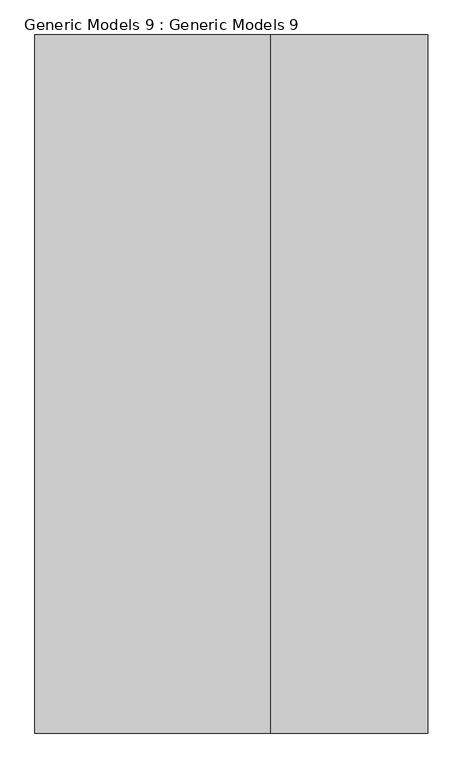
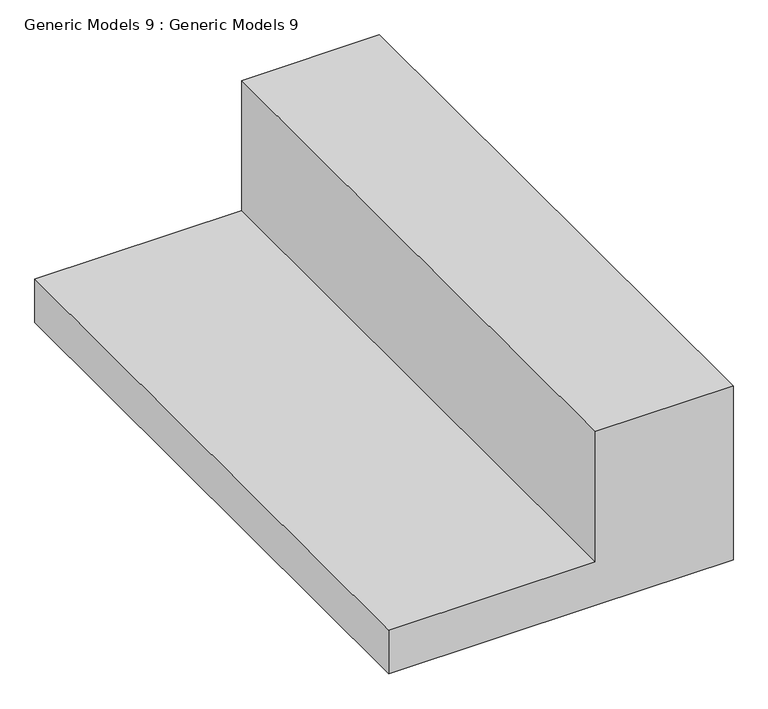
"""IFC4 building model written with IfcOpenShell, lengths in millimetres: proxy geometry, Generic Models 9 : Generic Models 9."""

from ifc_helpers import new_model, si_unit, frame, origin, place, context, project, spatial, polyline, outline, extrude, source, transform, mapped, element, save


def generic_models_9_generic_models_9_4d3f9729(model_context):
    return source(origin(), model_context, "Body", "SweptSolid", [
        extrude(outline(polyline([(3657.6, -12121.2371373), (3962.4, -12121.2371373), (3962.4, -12349.8371373), (3733.8, -12349.8371373), (3733.8, -12692.7371373), (3657.6, -12692.7371373), (3657.6, -12349.8371373), (3657.6, -12121.2371373)])), frame((0.0, -3532.661407, 0.0), z_axis=(0.0, 1.0, 0.0), x_axis=(0.0, 0.0, 1.0)), (0.0, 0.0, 1.0), 1016.0),
    ])


if __name__ == "__main__":
    model = new_model("IFC4")
    model_context = context("Model", 3, world=origin())
    ifc_project = project(units=[si_unit("LENGTHUNIT", "METRE", prefix="MILLI")], contexts=[model_context])
    site = spatial("IfcSite", under=ifc_project)
    building = spatial("IfcBuilding", under=site)
    placement = place(None, origin())
    generic_models_9_generic_models_9_shape = generic_models_9_generic_models_9_4d3f9729(model_context)
    element("IfcBuildingElementProxy", 1, Name="Generic Models 9 : Generic Models 9", ObjectType="Generic Models 9 : Generic Models 9", at=placement, inside=building, context=model_context, shape_type="MappedRepresentation", body=[
        mapped(generic_models_9_generic_models_9_shape, transform((0.0, 0.0, 0.0), x_axis=(1.0, 0.0, 0.0), y_axis=(0.0, 1.0, 0.0), z_axis=(0.0, 0.0, 1.0))),
    ])
    save(model, "model.ifc")

# Revit data of these elements
# Element 1 (IfcBuildingElementProxy, "Generic Models 9 : Generic Models 9")
#   Materials on its faces: "Gypsum Wall Board"
# Materials
#   "Gypsum Wall Board": class "Generic", colour RGB 127 127 127, transparency 0, Description = "Gypsum Wall Board", Cost = 0
